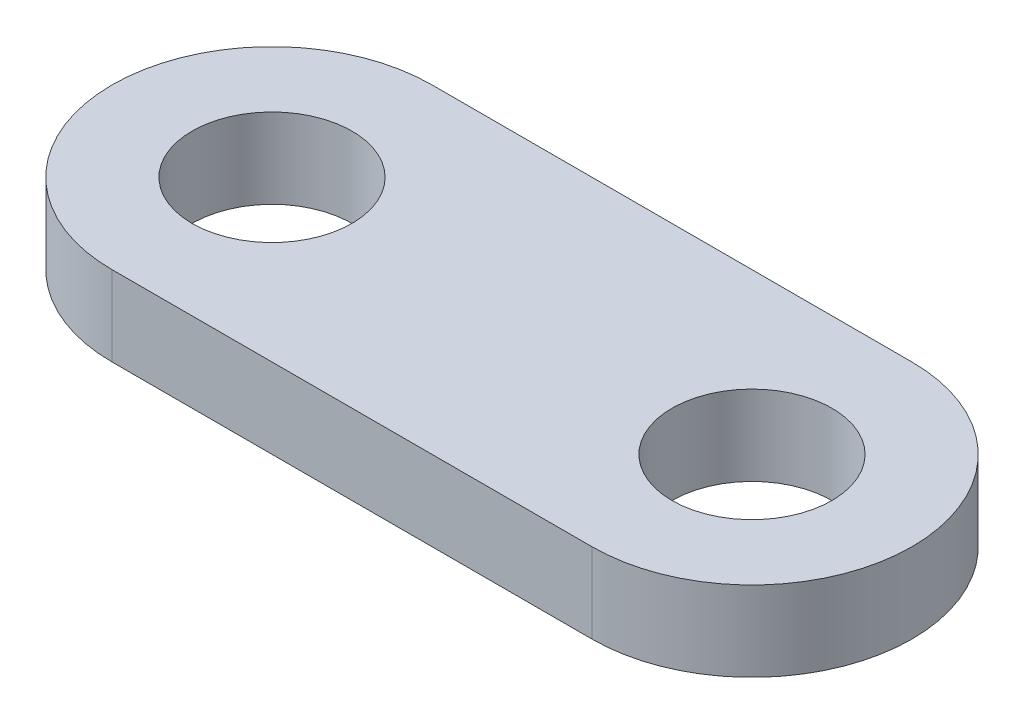
ISO-10303-21;
HEADER;
FILE_DESCRIPTION(('STEP AP214'),'2;1');
FILE_NAME('part.step','',(''),(''),'','','');
FILE_SCHEMA(('AUTOMOTIVE_DESIGN { 1 0 10303 214 1 1 1 1 }'));
ENDSEC;
DATA;
#1=APPLICATION_CONTEXT('core data for automotive mechanical design processes');
#2=APPLICATION_PROTOCOL_DEFINITION('international standard','automotive_design',2000,#1);
#3=PRODUCT_CONTEXT('',#1,'mechanical');
#4=PRODUCT('Part','Part','',(#3));
#5=PRODUCT_RELATED_PRODUCT_CATEGORY('part','',(#4));
#6=PRODUCT_DEFINITION_FORMATION('','',#4);
#7=PRODUCT_DEFINITION_CONTEXT('part definition',#1,'design');
#8=PRODUCT_DEFINITION('design','',#6,#7);
#9=PRODUCT_DEFINITION_SHAPE('','',#8);
#10=(LENGTH_UNIT() NAMED_UNIT(*) SI_UNIT(.MILLI.,.METRE.));
#11=(NAMED_UNIT(*) PLANE_ANGLE_UNIT() SI_UNIT($,.RADIAN.));
#12=(NAMED_UNIT(*) SI_UNIT($,.STERADIAN.) SOLID_ANGLE_UNIT());
#13=UNCERTAINTY_MEASURE_WITH_UNIT(LENGTH_MEASURE(1.E-05),#10,'distance_accuracy_value','');
#14=(GEOMETRIC_REPRESENTATION_CONTEXT(3) GLOBAL_UNCERTAINTY_ASSIGNED_CONTEXT((#13)) GLOBAL_UNIT_ASSIGNED_CONTEXT((#10,
#11,#12)) REPRESENTATION_CONTEXT('',''));
#15=CARTESIAN_POINT('',(0.,0.,0.));
#16=DIRECTION('',(0.,0.,1.));
#17=DIRECTION('',(1.,0.,0.));
#18=AXIS2_PLACEMENT_3D('',#15,#16,#17);
#19=CARTESIAN_POINT('',(-15.,5.,0.));
#20=DIRECTION('',(0.,1.,0.));
#21=DIRECTION('',(0.,0.,1.));
#22=AXIS2_PLACEMENT_3D('',#19,#20,#21);
#23=PLANE('',#22);
#24=CARTESIAN_POINT('',(-15.,5.,0.));
#25=DIRECTION('',(0.,1.,0.));
#26=DIRECTION('',(0.,0.,1.));
#27=AXIS2_PLACEMENT_3D('',#24,#25,#26);
#28=CIRCLE('',#27,5.);
#29=CARTESIAN_POINT('',(-15.,5.,5.));
#30=VERTEX_POINT('',#29);
#31=EDGE_CURVE('E106',#30,#30,#28,.T.);
#32=ORIENTED_EDGE('',*,*,#31,.F.);
#33=EDGE_LOOP('',(#32));
#34=FACE_BOUND('',#33,.T.);
#35=CARTESIAN_POINT('',(-15.,5.,0.));
#36=DIRECTION('',(0.,1.,0.));
#37=DIRECTION('',(0.,0.,1.));
#38=AXIS2_PLACEMENT_3D('',#35,#36,#37);
#39=CIRCLE('',#38,10.);
#40=CARTESIAN_POINT('',(-15.,5.,-10.));
#41=VERTEX_POINT('',#40);
#42=CARTESIAN_POINT('',(-15.,5.,10.));
#43=VERTEX_POINT('',#42);
#44=EDGE_CURVE('E93',#41,#43,#39,.T.);
#45=ORIENTED_EDGE('',*,*,#44,.T.);
#46=DIRECTION('',(1.,0.,0.));
#47=VECTOR('',#46,1.);
#48=CARTESIAN_POINT('',(-15.,5.,10.));
#49=LINE('',#48,#47);
#50=CARTESIAN_POINT('',(15.,5.,10.));
#51=VERTEX_POINT('',#50);
#52=EDGE_CURVE('E88',#43,#51,#49,.T.);
#53=ORIENTED_EDGE('',*,*,#52,.T.);
#54=CARTESIAN_POINT('',(15.,5.,0.));
#55=DIRECTION('',(0.,1.,0.));
#56=DIRECTION('',(0.,0.,1.));
#57=AXIS2_PLACEMENT_3D('',#54,#55,#56);
#58=CIRCLE('',#57,10.);
#59=CARTESIAN_POINT('',(15.,5.,-10.));
#60=VERTEX_POINT('',#59);
#61=EDGE_CURVE('E90',#51,#60,#58,.T.);
#62=ORIENTED_EDGE('',*,*,#61,.T.);
#63=DIRECTION('',(-1.,0.,0.));
#64=VECTOR('',#63,1.);
#65=CARTESIAN_POINT('',(-15.,5.,-10.));
#66=LINE('',#65,#64);
#67=EDGE_CURVE('E57',#60,#41,#66,.T.);
#68=ORIENTED_EDGE('',*,*,#67,.T.);
#69=EDGE_LOOP('',(#45,#53,#62,#68));
#70=FACE_BOUND('',#69,.T.);
#71=CARTESIAN_POINT('',(15.,5.,0.));
#72=DIRECTION('',(0.,1.,0.));
#73=DIRECTION('',(0.,0.,1.));
#74=AXIS2_PLACEMENT_3D('',#71,#72,#73);
#75=CIRCLE('',#74,5.);
#76=CARTESIAN_POINT('',(15.,5.,5.));
#77=VERTEX_POINT('',#76);
#78=EDGE_CURVE('E122',#77,#77,#75,.T.);
#79=ORIENTED_EDGE('',*,*,#78,.F.);
#80=EDGE_LOOP('',(#79));
#81=FACE_BOUND('',#80,.T.);
#82=ADVANCED_FACE('F39',(#34,#70,#81),#23,.T.);
#83=CARTESIAN_POINT('',(-15.,0.,0.));
#84=DIRECTION('',(0.,1.,0.));
#85=DIRECTION('',(0.,0.,1.));
#86=AXIS2_PLACEMENT_3D('',#83,#84,#85);
#87=PLANE('',#86);
#88=CARTESIAN_POINT('',(-15.,0.,0.));
#89=DIRECTION('',(0.,1.,0.));
#90=DIRECTION('',(0.,0.,1.));
#91=AXIS2_PLACEMENT_3D('',#88,#89,#90);
#92=CIRCLE('',#91,10.);
#93=CARTESIAN_POINT('',(-15.,0.,-10.));
#94=VERTEX_POINT('',#93);
#95=CARTESIAN_POINT('',(-15.,0.,10.));
#96=VERTEX_POINT('',#95);
#97=EDGE_CURVE('E103',#94,#96,#92,.T.);
#98=ORIENTED_EDGE('',*,*,#97,.F.);
#99=DIRECTION('',(-1.,0.,0.));
#100=VECTOR('',#99,1.);
#101=CARTESIAN_POINT('',(-15.,0.,-10.));
#102=LINE('',#101,#100);
#103=CARTESIAN_POINT('',(15.,0.,-10.));
#104=VERTEX_POINT('',#103);
#105=EDGE_CURVE('E76',#104,#94,#102,.T.);
#106=ORIENTED_EDGE('',*,*,#105,.F.);
#107=CARTESIAN_POINT('',(15.,0.,0.));
#108=DIRECTION('',(0.,1.,0.));
#109=DIRECTION('',(0.,0.,1.));
#110=AXIS2_PLACEMENT_3D('',#107,#108,#109);
#111=CIRCLE('',#110,10.);
#112=CARTESIAN_POINT('',(15.,0.,10.));
#113=VERTEX_POINT('',#112);
#114=EDGE_CURVE('E71',#113,#104,#111,.T.);
#115=ORIENTED_EDGE('',*,*,#114,.F.);
#116=DIRECTION('',(1.,0.,0.));
#117=VECTOR('',#116,1.);
#118=CARTESIAN_POINT('',(-15.,0.,10.));
#119=LINE('',#118,#117);
#120=EDGE_CURVE('E92',#96,#113,#119,.T.);
#121=ORIENTED_EDGE('',*,*,#120,.F.);
#122=EDGE_LOOP('',(#98,#106,#115,#121));
#123=FACE_BOUND('',#122,.T.);
#124=CARTESIAN_POINT('',(-15.,0.,0.));
#125=DIRECTION('',(0.,1.,0.));
#126=DIRECTION('',(0.,0.,1.));
#127=AXIS2_PLACEMENT_3D('',#124,#125,#126);
#128=CIRCLE('',#127,5.);
#129=CARTESIAN_POINT('',(-15.,0.,5.));
#130=VERTEX_POINT('',#129);
#131=EDGE_CURVE('E119',#130,#130,#128,.T.);
#132=ORIENTED_EDGE('',*,*,#131,.T.);
#133=EDGE_LOOP('',(#132));
#134=FACE_BOUND('',#133,.T.);
#135=CARTESIAN_POINT('',(15.,0.,0.));
#136=DIRECTION('',(0.,1.,0.));
#137=DIRECTION('',(0.,0.,1.));
#138=AXIS2_PLACEMENT_3D('',#135,#136,#137);
#139=CIRCLE('',#138,5.);
#140=CARTESIAN_POINT('',(15.,0.,5.));
#141=VERTEX_POINT('',#140);
#142=EDGE_CURVE('E121',#141,#141,#139,.T.);
#143=ORIENTED_EDGE('',*,*,#142,.T.);
#144=EDGE_LOOP('',(#143));
#145=FACE_BOUND('',#144,.T.);
#146=ADVANCED_FACE('F111',(#123,#134,#145),#87,.F.);
#147=CARTESIAN_POINT('',(-15.,5.,0.));
#148=DIRECTION('',(0.,-1.,0.));
#149=DIRECTION('',(0.,0.,-1.));
#150=AXIS2_PLACEMENT_3D('',#147,#148,#149);
#151=CYLINDRICAL_SURFACE('',#150,10.);
#152=ORIENTED_EDGE('',*,*,#97,.T.);
#153=DIRECTION('',(0.,-1.,0.));
#154=VECTOR('',#153,1.);
#155=CARTESIAN_POINT('',(-15.,5.,10.));
#156=LINE('',#155,#154);
#157=EDGE_CURVE('E11',#43,#96,#156,.T.);
#158=ORIENTED_EDGE('',*,*,#157,.F.);
#159=ORIENTED_EDGE('',*,*,#44,.F.);
#160=DIRECTION('',(0.,-1.,0.));
#161=VECTOR('',#160,1.);
#162=CARTESIAN_POINT('',(-15.,5.,-10.));
#163=LINE('',#162,#161);
#164=EDGE_CURVE('E97',#41,#94,#163,.T.);
#165=ORIENTED_EDGE('',*,*,#164,.T.);
#166=EDGE_LOOP('',(#152,#158,#159,#165));
#167=FACE_BOUND('',#166,.T.);
#168=ADVANCED_FACE('F41',(#167),#151,.T.);
#169=CARTESIAN_POINT('',(-15.,5.,10.));
#170=DIRECTION('',(0.,0.,-1.));
#171=DIRECTION('',(-1.,0.,0.));
#172=AXIS2_PLACEMENT_3D('',#169,#170,#171);
#173=PLANE('',#172);
#174=ORIENTED_EDGE('',*,*,#120,.T.);
#175=DIRECTION('',(0.,-1.,0.));
#176=VECTOR('',#175,1.);
#177=CARTESIAN_POINT('',(15.,5.,10.));
#178=LINE('',#177,#176);
#179=EDGE_CURVE('E48',#51,#113,#178,.T.);
#180=ORIENTED_EDGE('',*,*,#179,.F.);
#181=ORIENTED_EDGE('',*,*,#52,.F.);
#182=ORIENTED_EDGE('',*,*,#157,.T.);
#183=EDGE_LOOP('',(#174,#180,#181,#182));
#184=FACE_BOUND('',#183,.T.);
#185=ADVANCED_FACE('F94',(#184),#173,.F.);
#186=CARTESIAN_POINT('',(15.,5.,0.));
#187=DIRECTION('',(0.,-1.,0.));
#188=DIRECTION('',(0.,0.,-1.));
#189=AXIS2_PLACEMENT_3D('',#186,#187,#188);
#190=CYLINDRICAL_SURFACE('',#189,10.);
#191=ORIENTED_EDGE('',*,*,#114,.T.);
#192=DIRECTION('',(0.,-1.,0.));
#193=VECTOR('',#192,1.);
#194=CARTESIAN_POINT('',(15.,5.,-10.));
#195=LINE('',#194,#193);
#196=EDGE_CURVE('E96',#60,#104,#195,.T.);
#197=ORIENTED_EDGE('',*,*,#196,.F.);
#198=ORIENTED_EDGE('',*,*,#61,.F.);
#199=ORIENTED_EDGE('',*,*,#179,.T.);
#200=EDGE_LOOP('',(#191,#197,#198,#199));
#201=FACE_BOUND('',#200,.T.);
#202=ADVANCED_FACE('F100',(#201),#190,.T.);
#203=CARTESIAN_POINT('',(-15.,5.,-10.));
#204=DIRECTION('',(0.,0.,1.));
#205=DIRECTION('',(1.,0.,0.));
#206=AXIS2_PLACEMENT_3D('',#203,#204,#205);
#207=PLANE('',#206);
#208=ORIENTED_EDGE('',*,*,#105,.T.);
#209=ORIENTED_EDGE('',*,*,#164,.F.);
#210=ORIENTED_EDGE('',*,*,#67,.F.);
#211=ORIENTED_EDGE('',*,*,#196,.T.);
#212=EDGE_LOOP('',(#208,#209,#210,#211));
#213=FACE_BOUND('',#212,.T.);
#214=ADVANCED_FACE('F112',(#213),#207,.F.);
#215=CARTESIAN_POINT('',(-15.,5.,0.));
#216=DIRECTION('',(0.,-1.,0.));
#217=DIRECTION('',(0.,0.,-1.));
#218=AXIS2_PLACEMENT_3D('',#215,#216,#217);
#219=CYLINDRICAL_SURFACE('',#218,5.);
#220=ORIENTED_EDGE('',*,*,#31,.T.);
#221=EDGE_LOOP('',(#220));
#222=FACE_BOUND('',#221,.T.);
#223=ORIENTED_EDGE('',*,*,#131,.F.);
#224=EDGE_LOOP('',(#223));
#225=FACE_BOUND('',#224,.T.);
#226=ADVANCED_FACE('F143',(#222,#225),#219,.F.);
#227=CARTESIAN_POINT('',(15.,5.,0.));
#228=DIRECTION('',(0.,-1.,0.));
#229=DIRECTION('',(0.,0.,-1.));
#230=AXIS2_PLACEMENT_3D('',#227,#228,#229);
#231=CYLINDRICAL_SURFACE('',#230,5.);
#232=ORIENTED_EDGE('',*,*,#78,.T.);
#233=EDGE_LOOP('',(#232));
#234=FACE_BOUND('',#233,.T.);
#235=ORIENTED_EDGE('',*,*,#142,.F.);
#236=EDGE_LOOP('',(#235));
#237=FACE_BOUND('',#236,.T.);
#238=ADVANCED_FACE('F128',(#234,#237),#231,.F.);
#239=CLOSED_SHELL('',(#82,#146,#168,#185,#202,#214,#226,#238));
#240=MANIFOLD_SOLID_BREP('B2',#239);
#241=ADVANCED_BREP_SHAPE_REPRESENTATION('',(#18,#240),#14);
#242=SHAPE_DEFINITION_REPRESENTATION(#9,#241);
ENDSEC;
END-ISO-10303-21;
